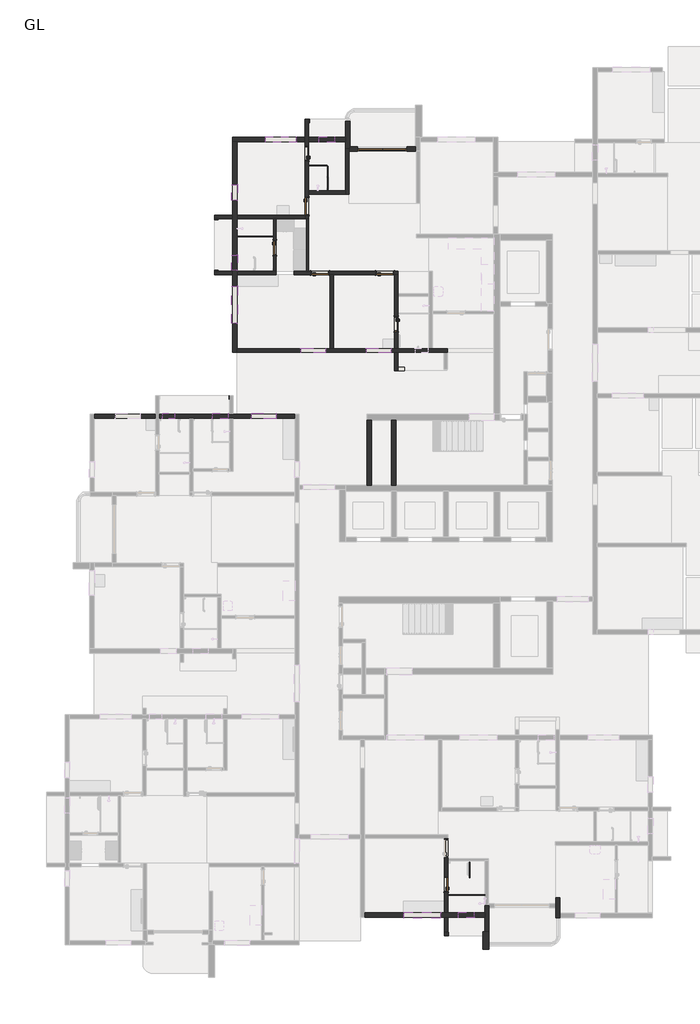
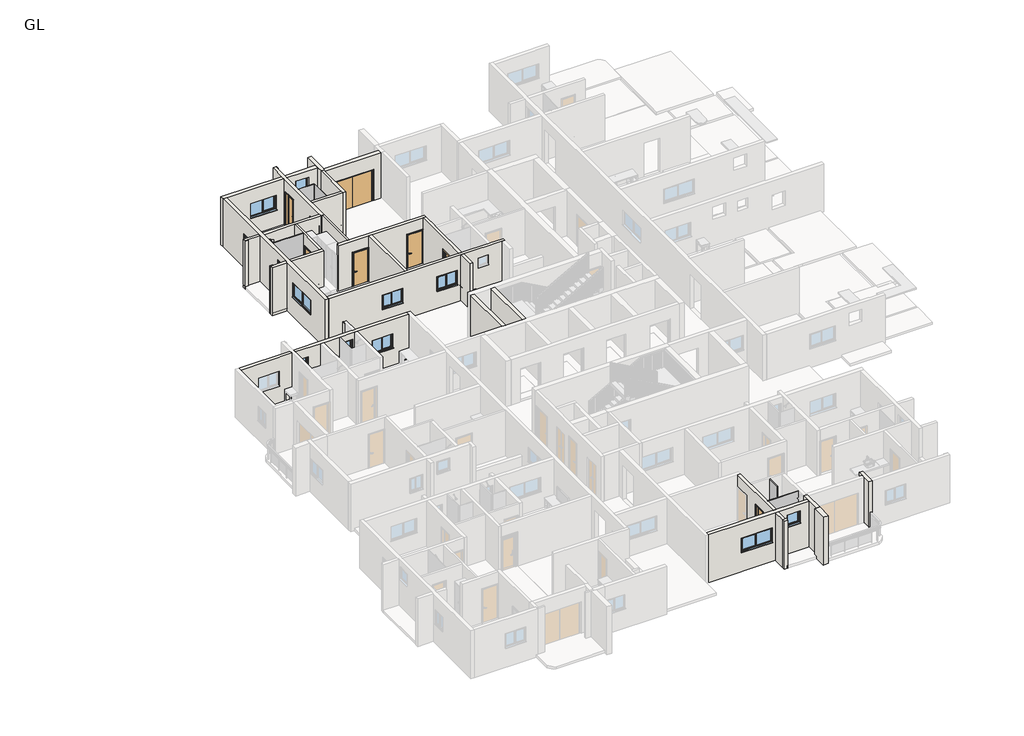
# One storey, part 3 of 14: 30 walls, 12 windows, 8 doors, 5 plates.
"""IFC4 building model written with IfcOpenShell, lengths in millimetres."""

from ifc_helpers import new_model, si_unit, frame, origin, origin_with_axes, place, context, project, spatial, polyline, outline, extrude, faceted_brep, transform, mapped, element, save
from components import doors_concept_extdbl_8_449e5563, doors_intsgl_2_5_door_ce04bd24, doors_intsgl_2_5_door_1f5f3f16, doors_intsgl_2_5_door_57e365e7, doors_intsgl_2_5_door_fd097d29, doors_intsgl_3_door_8261d8fb, system_panel_glazed_7a21471d, system_panel_glazed_bd0dc997, system_panel_glazed_f5f8a0d0, system_panel_glazed_29ba505a, system_panel_glazed_fbb400a4, windows_dbl_plain_2_5_5b7baf13, windows_dbl_plain_4_e08ba9e4, windows_dbl_plain_4_44133fe2, windows_dbl_plain_5_e9a2d570, windows_dbl_plain_6_3da2432f, windows_dbl_plain_6_22e4277a, windows_sgl_plain_2_82341a49, windows_sgl_plain_2_5_9e76a6e6, windows_sgl_plain_2_5_21186da1, windows_sgl_plain_2_5_1233c963

model = new_model("IFC4")

# Units and contexts
model_context = context("Model", 3, world=origin())
ifc_project = project(units=[si_unit("LENGTHUNIT", "METRE", prefix="MILLI")], contexts=[model_context])

# Site, building, storey
site = spatial("IfcSite", under=ifc_project)
building = spatial("IfcBuilding", under=site)
storey = spatial("IfcBuildingStorey", under=building, Name="GL", Elevation=0.0)

# Doors
placement = place(None, origin())
doors_concept_extdbl_8_shape = doors_concept_extdbl_8_449e5563(model_context)
element("IfcDoor", 1, ObjectType="Doors_Concept_ExtDbl : 8'", at=placement, inside=storey, context=model_context, shape_type="MappedRepresentation", body=[
    mapped(doors_concept_extdbl_8_shape, transform((-1155.7878137, 95616.8756254, 0.0), x_axis=(-1.0, 0.0, 0.0), y_axis=(0.0, -1.0, 0.0), z_axis=(0.0, 0.0, 1.0))),
])
doors_intsgl_2_5_door_shape = doors_intsgl_2_5_door_ce04bd24(model_context)
element("IfcDoor", 2, ObjectType="Doors_IntSgl : 2.5' DOOR", at=placement, inside=storey, context=model_context, shape_type="MappedRepresentation", body=[
    mapped(doors_intsgl_2_5_door_shape, transform((-457.962999, 86931.0916254, 149.9616), x_axis=(0.0, -1.0, 0.0), y_axis=(1.0, 0.0, 0.0), z_axis=(0.0, 0.0, 1.0))),
])
doors_intsgl_2_5_door_2_shape = doors_intsgl_2_5_door_1f5f3f16(model_context)
element("IfcDoor", 3, ObjectType="Doors_IntSgl : 2.5' DOOR", at=placement, inside=storey, context=model_context, shape_type="MappedRepresentation", body=[
    mapped(doors_intsgl_2_5_door_2_shape, transform((-6490.3162192, 90712.3517744, 149.9616), x_axis=(0.0, -1.0, 0.0), y_axis=(1.0, 0.0, 0.0), z_axis=(0.0, 0.0, 1.0))),
])
doors_intsgl_2_5_door_3_shape = doors_intsgl_2_5_door_57e365e7(model_context)
element("IfcDoor", 4, ObjectType="Doors_IntSgl : 2.5' DOOR", at=placement, inside=storey, context=model_context, shape_type="MappedRepresentation", body=[
    mapped(doors_intsgl_2_5_door_3_shape, transform((2014.4093567, 59142.1083045, 149.9616), x_axis=(0.0, 1.0, 0.0), y_axis=(-1.0, 0.0, 0.0), z_axis=(0.0, 0.0, 1.0))),
])
doors_intsgl_2_5_door_4_shape = doors_intsgl_2_5_door_fd097d29(model_context)
element("IfcDoor", 5, ObjectType="Doors_IntSgl : 2.5' DOOR", at=placement, inside=storey, context=model_context, shape_type="MappedRepresentation", body=[
    mapped(doors_intsgl_2_5_door_4_shape, transform((-4892.1482192, 95388.5507225, 149.9616), x_axis=(0.0, 1.0, 0.0), y_axis=(-1.0, 0.0, 0.0), z_axis=(0.0, 0.0, 1.0))),
])
doors_intsgl_3_door_shape = doors_intsgl_3_door_8261d8fb(model_context)
element("IfcDoor", 6, ObjectType="Doors_IntSgl : 3' DOOR", at=placement, inside=storey, context=model_context, shape_type="MappedRepresentation", body=[
    mapped(doors_intsgl_3_door_shape, transform((-1027.430999, 89469.7837744, 149.9616), x_axis=(1.0, 0.0, 0.0), y_axis=(0.0, 1.0, 0.0), z_axis=(0.0, 0.0, 1.0))),
])
element("IfcDoor", 7, ObjectType="Doors_IntSgl : 3' DOOR", at=placement, inside=storey, context=model_context, shape_type="MappedRepresentation", body=[
    mapped(doors_intsgl_3_door_shape, transform((-4246.4802192, 89469.7837744, 149.9616), x_axis=(1.0, 0.0, 0.0), y_axis=(0.0, 1.0, 0.0), z_axis=(0.0, 0.0, 1.0))),
])
element("IfcDoor", 8, ObjectType="Doors_IntSgl : 3' DOOR", at=placement, inside=storey, context=model_context, shape_type="MappedRepresentation", body=[
    mapped(doors_intsgl_3_door_shape, transform((-4892.1482192, 92780.648129, 149.9616), x_axis=(0.0, -1.0, 0.0), y_axis=(1.0, 0.0, 0.0), z_axis=(0.0, 0.0, 1.0))),
])

# Plates
system_panel_glazed_shape = system_panel_glazed_7a21471d(model_context)
element("IfcPlate", 9, ObjectType="System Panel : Glazed", at=placement, inside=storey, context=model_context, shape_type="MappedRepresentation", body=[
    mapped(system_panel_glazed_shape, transform((3014.0263567, 58649.9833045, 0.0), x_axis=(-1.0, 0.0, 0.0), y_axis=(0.0, -1.0, 0.0), z_axis=(0.0, 0.0, 1.0))),
])
system_panel_glazed_2_shape = system_panel_glazed_bd0dc997(model_context)
element("IfcPlate", 10, ObjectType="System Panel : Glazed", at=placement, inside=storey, context=model_context, shape_type="MappedRepresentation", body=[
    mapped(system_panel_glazed_2_shape, transform((3149.1144026, 59856.6583045, 0.0), x_axis=(0.0, -1.0, 0.0), y_axis=(1.0, 0.0, 0.0), z_axis=(0.0, 0.0, 1.0))),
])
system_panel_glazed_3_shape = system_panel_glazed_f5f8a0d0(model_context)
element("IfcPlate", 11, ObjectType="System Panel : Glazed", at=placement, inside=storey, context=model_context, shape_type="MappedRepresentation", body=[
    mapped(system_panel_glazed_3_shape, transform((-7453.4306091, 91235.312129, 0.0), x_axis=(1.0, 0.0, 0.0), y_axis=(0.0, 1.0, 0.0), z_axis=(0.0, 0.0, 1.0))),
])
system_panel_glazed_4_shape = system_panel_glazed_29ba505a(model_context)
element("IfcPlate", 12, ObjectType="System Panel : Glazed", at=placement, inside=storey, context=model_context, shape_type="MappedRepresentation", body=[
    mapped(system_panel_glazed_4_shape, transform((-4348.0802192, 94755.9639277, 0.0), x_axis=(1.0, 0.0, 0.0), y_axis=(0.0, 1.0, 0.0), z_axis=(0.0, 0.0, 1.0))),
])
system_panel_glazed_5_shape = system_panel_glazed_fbb400a4(model_context)
element("IfcPlate", 13, ObjectType="System Panel : Glazed", at=placement, inside=storey, context=model_context, shape_type="MappedRepresentation", body=[
    mapped(system_panel_glazed_5_shape, transform((-3890.8802192, 94151.5180788, 0.0), x_axis=(0.0, -1.0, 0.0), y_axis=(1.0, 0.0, 0.0), z_axis=(0.0, 0.0, 1.0))),
])

# Walls
element("IfcWall", 14, ObjectType="W2", at=placement, inside=storey, context=model_context, shape_type="Brep", body=[
    faceted_brep([(-2987.294999, 95616.8756254, 0.0), (-2987.294999, 93547.0722299, 0.0), (-2987.294999, 93373.3362299, 0.0), (-2987.294999, 93373.3362299, 3000.0), (-2987.294999, 93547.0722299, 3000.0), (-2987.294999, 95616.8756254, 3000.0), (-2813.558999, 95616.8756254, 0.0), (-2813.558999, 95616.8756254, 3000.0), (-2813.558999, 95510.1956254, 3000.0), (-2813.558999, 93373.3362299, 3000.0), (-2813.558999, 93373.3362299, 0.0), (-2813.558999, 95510.1956254, 0.0)], [[[0, 1, 2, 3, 4, 5]], [[6, 7, 8, 9, 10, 11]], [[2, 1, 0, 6, 11, 10]], [[5, 4, 3, 9, 8, 7]], [[0, 5, 7, 6]], [[3, 2, 10, 9]]]),
])
element("IfcWall", 15, ObjectType="W2", at=placement, inside=storey, context=model_context, shape_type="Brep", body=[
    faceted_brep([(-4979.0162192, 97086.2867225, 0.0), (-4979.0162192, 96193.4556254, 0.0), (-4979.0162192, 95964.8556254, 0.0), (-4979.0162192, 92323.448129, 0.0), (-4979.0162192, 92149.712129, 0.0), (-4979.0162192, 92149.712129, 3000.0), (-4979.0162192, 92323.448129, 3000.0), (-4979.0162192, 95964.8556254, 3000.0), (-4979.0162192, 96193.4556254, 3000.0), (-4979.0162192, 97086.2867225, 3000.0), (-4979.0162192, 92323.448129, 2259.9616), (-4979.0162192, 92323.448129, 149.9616), (-4979.0162192, 93237.848129, 149.9616), (-4979.0162192, 93237.848129, 2259.9616), (-4979.0162192, 95769.5507225, 149.9616), (-4979.0162192, 95769.5507225, 2259.9616), (-4979.0162192, 95007.5507225, 2259.9616), (-4979.0162192, 95007.5507225, 149.9616), (-4805.2802192, 92149.712129, 0.0), (-4805.2802192, 93373.3362299, 0.0), (-4805.2802192, 93547.0722299, 0.0), (-4805.2802192, 95964.8556254, 0.0), (-4805.2802192, 96193.4556254, 0.0), (-4805.2802192, 96912.5507225, 0.0), (-4805.2802192, 97086.2867225, 0.0), (-4805.2802192, 97086.2867225, 3000.0), (-4805.2802192, 96912.5507225, 3000.0), (-4805.2802192, 96193.4556254, 3000.0), (-4805.2802192, 95964.8556254, 3000.0), (-4805.2802192, 93547.0722299, 3000.0), (-4805.2802192, 93373.3362299, 3000.0), (-4805.2802192, 92149.712129, 3000.0), (-4805.2802192, 92323.448129, 149.9616), (-4805.2802192, 92323.448129, 2259.9616), (-4805.2802192, 93237.848129, 2259.9616), (-4805.2802192, 93237.848129, 149.9616), (-4805.2802192, 95769.5507225, 2259.9616), (-4805.2802192, 95769.5507225, 149.9616), (-4805.2802192, 95007.5507225, 149.9616), (-4805.2802192, 95007.5507225, 2259.9616), (-4919.5802192, 92149.712129, 0.0), (-4919.5802192, 92149.712129, 3000.0)], [[[0, 1, 2, 3, 4, 5, 6, 7, 8, 9], [10, 11, 12, 13], [14, 15, 16, 17]], [[18, 19, 20, 21, 22, 23, 24, 25, 26, 27, 28, 29, 30, 31], [32, 33, 34, 35], [36, 37, 38, 39]], [[4, 3, 2, 1, 0, 24, 23, 22, 21, 20, 19, 18, 40]], [[9, 8, 7, 6, 5, 41, 31, 30, 29, 28, 27, 26, 25]], [[5, 4, 40, 18, 31, 41]], [[0, 9, 25, 24]], [[32, 11, 10, 33]], [[33, 10, 13, 34]], [[34, 13, 12, 35]], [[11, 32, 35, 12]], [[14, 37, 36, 15]], [[15, 36, 39, 16]], [[38, 17, 16, 39]], [[37, 14, 17, 38]]]),
])
element("IfcWall", 16, ObjectType="W2", at=placement, inside=storey, context=model_context, shape_type="Brep", body=[
    faceted_brep([(-8359.394999, 85538.1556254, 0.0), (-538.480999, 85538.1556254, 0.0), (-364.744999, 85538.1556254, 0.0), (1899.919001, 85538.1556254, 0.0), (2073.655001, 85538.1556254, 0.0), (2080.005001, 85538.1556254, 0.0), (2080.005001, 85538.1556254, 1171.2), (2080.005001, 85538.1556254, 3000.0), (2073.655001, 85538.1556254, 3000.0), (1899.919001, 85538.1556254, 3000.0), (-364.744999, 85538.1556254, 3000.0), (-538.480999, 85538.1556254, 3000.0), (-8359.394999, 85538.1556254, 3000.0), (-3962.5906208, 85538.1556254, 2110.0), (-3962.5906208, 85538.1556254, 1200.0), (-5181.7906208, 85538.1556254, 1200.0), (-5181.7906208, 85538.1556254, 2110.0), (-722.630999, 85538.1556254, 2110.0), (-722.630999, 85538.1556254, 1200.0), (-1941.830999, 85538.1556254, 1200.0), (-1941.830999, 85538.1556254, 2110.0), (1106.169001, 85538.1556254, 2438.4), (1106.169001, 85538.1556254, 1828.8), (496.569001, 85538.1556254, 1828.8), (496.569001, 85538.1556254, 2438.4), (-8359.394999, 85711.8916254, 0.0), (-8359.394999, 85711.8916254, 3000.0), (-3759.3906208, 85711.8916254, 3000.0), (-3585.6546208, 85711.8916254, 3000.0), (-544.830999, 85711.8916254, 3000.0), (-371.094999, 85711.8916254, 3000.0), (1156.969001, 85711.8916254, 3000.0), (1330.705001, 85711.8916254, 3000.0), (2080.005001, 85711.8916254, 3000.0), (2080.005001, 85711.8916254, 1171.2), (2080.005001, 85711.8916254, 0.0), (1330.705001, 85711.8916254, 0.0), (1156.969001, 85711.8916254, 0.0), (-371.094999, 85711.8916254, 0.0), (-544.830999, 85711.8916254, 0.0), (-3585.6546208, 85711.8916254, 0.0), (-3759.3906208, 85711.8916254, 0.0), (-3962.5906208, 85711.8916254, 2110.0), (-5181.7906208, 85711.8916254, 2110.0), (-5181.7906208, 85711.8916254, 1200.0), (-3962.5906208, 85711.8916254, 1200.0), (-722.630999, 85711.8916254, 2110.0), (-1941.830999, 85711.8916254, 2110.0), (-1941.830999, 85711.8916254, 1200.0), (-722.630999, 85711.8916254, 1200.0), (1106.169001, 85711.8916254, 2438.4), (496.569001, 85711.8916254, 2438.4), (496.569001, 85711.8916254, 1828.8), (1106.169001, 85711.8916254, 1828.8)], [[[0, 1, 2, 3, 4, 5, 6, 7, 8, 9, 10, 11, 12], [13, 14, 15, 16], [17, 18, 19, 20], [21, 22, 23, 24]], [[25, 26, 27, 28, 29, 30, 31, 32, 33, 34, 35, 36, 37, 38, 39, 40, 41], [42, 43, 44, 45], [46, 47, 48, 49], [50, 51, 52, 53]], [[5, 4, 3, 2, 1, 0, 25, 41, 40, 39, 38, 37, 36, 35]], [[7, 6, 5, 35, 34, 33]], [[12, 11, 10, 9, 8, 7, 33, 32, 31, 30, 29, 28, 27, 26]], [[0, 12, 26, 25]], [[14, 13, 42, 45]], [[15, 14, 45, 44]], [[16, 15, 44, 43]], [[13, 16, 43, 42]], [[18, 17, 46, 49]], [[19, 18, 49, 48]], [[20, 19, 48, 47]], [[17, 20, 47, 46]], [[22, 21, 50, 53]], [[23, 22, 53, 52]], [[24, 23, 52, 51]], [[21, 24, 51, 50]]]),
])
element("IfcWall", 17, ObjectType="W2", at=placement, inside=storey, context=model_context, shape_type="SweptSolid", body=[
    extrude(outline(polyline([(-4805.2802192, 93547.0722299), (-2987.294999, 93547.0722299), (-2987.294999, 93373.3362299), (-4805.2802192, 93373.3362299), (-4805.2802192, 93547.0722299)])), origin_with_axes(), (0.0, 0.0, 1.0), 3000.0),
])
element("IfcWall", 18, ObjectType="W2", at=placement, inside=storey, context=model_context, shape_type="Brep", body=[
    faceted_brep([(-4979.0162192, 92323.448129, 3000.0), (-4979.0162192, 92323.448129, 0.0), (-8359.394999, 92323.448129, 0.0), (-8359.394999, 92323.448129, 3000.0), (-4979.0162192, 92149.712129, 0.0), (-4979.0162192, 92149.712129, 3000.0), (-6433.1662192, 92149.712129, 3000.0), (-6547.4662192, 92149.712129, 3000.0), (-8359.394999, 92149.712129, 3000.0), (-8359.394999, 92149.712129, 0.0), (-6547.4662192, 92149.712129, 0.0), (-6433.1662192, 92149.712129, 0.0)], [[[0, 1, 2, 3]], [[4, 5, 6, 7, 8, 9, 10, 11]], [[1, 4, 11, 10, 9, 2]], [[5, 0, 3, 8, 7, 6]], [[1, 0, 5, 4]], [[3, 2, 9, 8]]]),
    faceted_brep([(-9487.5162192, 92323.448129, 0.0), (-9487.5162192, 92323.448129, 3000.0), (-8587.994999, 92323.448129, 3000.0), (-8587.994999, 92323.448129, 0.0), (-9487.5162192, 92149.712129, 3000.0), (-9487.5162192, 92149.712129, 0.0), (-9313.7802192, 92149.712129, 0.0), (-8587.994999, 92149.712129, 0.0), (-8587.994999, 92149.712129, 3000.0), (-9313.7802192, 92149.712129, 3000.0)], [[[0, 1, 2, 3]], [[4, 5, 6, 7, 8, 9]], [[5, 0, 3, 7, 6]], [[1, 4, 9, 8, 2]], [[3, 2, 8, 7]], [[1, 0, 5, 4]]]),
])
element("IfcWall", 19, ObjectType="W2", at=placement, inside=storey, context=model_context, shape_type="Brep", body=[
    faceted_brep([(-9487.5162192, 89382.9157744, 3000.0), (-9487.5162192, 89382.9157744, 0.0), (-8587.994999, 89382.9157744, 0.0), (-8587.994999, 89382.9157744, 3000.0), (-9487.5162192, 89556.6517744, 0.0), (-9487.5162192, 89556.6517744, 3000.0), (-9313.7802192, 89556.6517744, 3000.0), (-8587.994999, 89556.6517744, 3000.0), (-8587.994999, 89556.6517744, 0.0), (-9313.7802192, 89556.6517744, 0.0)], [[[0, 1, 2, 3]], [[4, 5, 6, 7, 8, 9]], [[1, 4, 9, 8, 2]], [[5, 0, 3, 7, 6]], [[3, 2, 8, 7]], [[1, 0, 5, 4]]]),
    faceted_brep([(-6433.1662192, 89382.9157744, 0.0), (-6433.1662192, 89382.9157744, 3000.0), (-8359.394999, 89382.9157744, 3000.0), (-8359.394999, 89382.9157744, 0.0), (-6433.1662192, 89556.6517744, 3000.0), (-6433.1662192, 89556.6517744, 0.0), (-6547.4662192, 89556.6517744, 0.0), (-8359.394999, 89556.6517744, 0.0), (-8359.394999, 89556.6517744, 3000.0), (-6547.4662192, 89556.6517744, 3000.0)], [[[0, 1, 2, 3]], [[4, 5, 6, 7, 8, 9]], [[5, 0, 3, 7, 6]], [[1, 4, 9, 8, 2]], [[3, 2, 8, 7]], [[1, 0, 5, 4]]]),
])
element("IfcWall", 20, ObjectType="W2", at=placement, inside=storey, context=model_context, shape_type="SweptSolid", body=[
    extrude(outline(polyline([(-9487.5162192, 92111.612129), (-9487.5162192, 92149.712129), (-9313.7802192, 92149.712129), (-9313.7802192, 92111.612129), (-9487.5162192, 92111.612129)])), origin_with_axes(), (0.0, 0.0, 1.0), 3000.0),
])
element("IfcWall", 21, ObjectType="W2", at=placement, inside=storey, context=model_context, shape_type="SweptSolid", body=[
    extrude(outline(polyline([(-9487.5162192, 89556.6517744), (-9487.5162192, 89601.1017744), (-9313.7802192, 89601.1017744), (-9313.7802192, 89556.6517744), (-9487.5162192, 89556.6517744)])), origin_with_axes(), (0.0, 0.0, 1.0), 3000.0),
])
element("IfcWall", 22, ObjectType="W2", at=placement, inside=storey, context=model_context, shape_type="Brep", body=[
    faceted_brep([(-5531.8235062, 89382.9157744, 0.0), (-3759.3906208, 89382.9157744, 0.0), (-3585.6546208, 89382.9157744, 0.0), (-544.830999, 89382.9157744, 0.0), (-371.094999, 89382.9157744, 0.0), (-371.094999, 89382.9157744, 3000.0), (-544.830999, 89382.9157744, 3000.0), (-3585.6546208, 89382.9157744, 3000.0), (-3759.3906208, 89382.9157744, 3000.0), (-5531.8235062, 89382.9157744, 3000.0), (-570.230999, 89382.9157744, 2259.9616), (-570.230999, 89382.9157744, 149.9616), (-1484.630999, 89382.9157744, 149.9616), (-1484.630999, 89382.9157744, 2259.9616), (-3789.2802192, 89382.9157744, 2259.9616), (-3789.2802192, 89382.9157744, 149.9616), (-4703.6802192, 89382.9157744, 149.9616), (-4703.6802192, 89382.9157744, 2259.9616), (-371.094999, 89556.6517744, 0.0), (-4805.2802192, 89556.6517744, 0.0), (-4919.5802192, 89556.6517744, 0.0), (-5531.8235062, 89556.6517744, 0.0), (-5531.8235062, 89556.6517744, 3000.0), (-4919.5802192, 89556.6517744, 3000.0), (-4805.2802192, 89556.6517744, 3000.0), (-371.094999, 89556.6517744, 3000.0), (-570.230999, 89556.6517744, 149.9616), (-570.230999, 89556.6517744, 2259.9616), (-1484.630999, 89556.6517744, 2259.9616), (-1484.630999, 89556.6517744, 149.9616), (-3789.2802192, 89556.6517744, 149.9616), (-3789.2802192, 89556.6517744, 2259.9616), (-4703.6802192, 89556.6517744, 2259.9616), (-4703.6802192, 89556.6517744, 149.9616)], [[[0, 1, 2, 3, 4, 5, 6, 7, 8, 9], [10, 11, 12, 13], [14, 15, 16, 17]], [[18, 19, 20, 21, 22, 23, 24, 25], [26, 27, 28, 29], [30, 31, 32, 33]], [[4, 3, 2, 1, 0, 21, 20, 19, 18]], [[9, 8, 7, 6, 5, 25, 24, 23, 22]], [[0, 9, 22, 21]], [[5, 4, 18, 25]], [[26, 11, 10, 27]], [[27, 10, 13, 28]], [[12, 29, 28, 13]], [[11, 26, 29, 12]], [[30, 15, 14, 31]], [[31, 14, 17, 32]], [[32, 17, 16, 33]], [[15, 30, 33, 16]]]),
])
element("IfcWall", 23, ObjectType="W2", at=placement, inside=storey, context=model_context, shape_type="SweptSolid", body=[
    extrude(outline(polyline([(-3585.6546208, 89382.9157744), (-3585.6546208, 85711.8916254), (-3759.3906208, 85711.8916254), (-3759.3906208, 89382.9157744), (-3585.6546208, 89382.9157744)])), origin_with_axes(), (0.0, 0.0, 1.0), 3000.0),
])
element("IfcWall", 24, ObjectType="W2", at=placement, inside=storey, context=model_context, shape_type="Brep", body=[
    faceted_brep([(-371.094999, 85711.8916254, 0.0), (-371.094999, 88321.7416254, 0.0), (-371.094999, 88436.0416254, 0.0), (-371.094999, 89382.9157744, 0.0), (-371.094999, 89382.9157744, 3000.0), (-371.094999, 88436.0416254, 3000.0), (-371.094999, 88321.7416254, 3000.0), (-371.094999, 85711.8916254, 3000.0), (-371.094999, 86550.0916254, 149.9616), (-371.094999, 86550.0916254, 2259.9616), (-371.094999, 87312.0916254, 2259.9616), (-371.094999, 87312.0916254, 149.9616), (-544.830999, 89382.9157744, 0.0), (-544.830999, 85711.8916254, 0.0), (-544.830999, 85711.8916254, 3000.0), (-544.830999, 89382.9157744, 3000.0), (-544.830999, 86550.0916254, 2259.9616), (-544.830999, 86550.0916254, 149.9616), (-544.830999, 87312.0916254, 149.9616), (-544.830999, 87312.0916254, 2259.9616)], [[[0, 1, 2, 3, 4, 5, 6, 7], [8, 9, 10, 11]], [[12, 13, 14, 15], [16, 17, 18, 19]], [[3, 2, 1, 0, 13, 12]], [[7, 6, 5, 4, 15, 14]], [[0, 7, 14, 13]], [[4, 3, 12, 15]], [[8, 17, 16, 9]], [[9, 16, 19, 10]], [[10, 19, 18, 11]], [[17, 8, 11, 18]]]),
])
element("IfcWall", 25, ObjectType="W2", at=placement, inside=storey, context=model_context, shape_type="Brep", body=[
    faceted_brep([(-538.480999, 85538.1556254, 0.0), (-538.480999, 84611.0556254, 0.0), (-538.480999, 84611.0556254, 3000.0), (-538.480999, 85538.1556254, 3000.0), (-364.744999, 85538.1556254, 0.0), (-364.744999, 85538.1556254, 3000.0), (-364.744999, 84611.0556254, 3000.0), (-364.744999, 84611.0556254, 1171.2), (-364.744999, 84611.0556254, 0.0), (-364.744999, 84784.7916254, 0.0)], [[[0, 1, 2, 3]], [[4, 5, 6, 7, 8, 9]], [[1, 0, 4, 9, 8]], [[3, 2, 6, 5]], [[0, 3, 5, 4]], [[2, 1, 8, 7, 6]]]),
])
element("IfcWall", 26, ObjectType="W2", at=placement, inside=storey, context=model_context, shape_type="SweptSolid", body=[
    extrude(outline(polyline([(-66.294999, 84611.0556254), (-364.744999, 84611.0556254), (-364.744999, 84784.7916254), (-66.294999, 84784.7916254), (-66.294999, 84611.0556254)])), origin_with_axes(), (0.0, 0.0, 1.0), 1171.2),
])
element("IfcWall", 27, ObjectType="W2", at=placement, inside=storey, context=model_context, shape_type="SweptSolid", body=[
    extrude(outline(polyline([(-8762.4991708, 83367.762856), (-8724.3991708, 83367.762856), (-8724.3991708, 83194.026856), (-8762.4991708, 83194.026856), (-8762.4991708, 83367.762856)])), origin_with_axes(), (0.0, 0.0, 1.0), 3000.0),
])
element("IfcWall", 28, ObjectType="W2", at=placement, inside=storey, context=model_context, shape_type="SweptSolid", body=[
    extrude(outline(polyline([(-4773.5302192, 96912.5507225), (-4805.2802192, 96912.5507225), (-4805.2802192, 97086.2867225), (-4773.5302192, 97086.2867225), (-4773.5302192, 96912.5507225)])), origin_with_axes(), (0.0, 0.0, 1.0), 3000.0),
])
element("IfcWall", 29, ObjectType="W2", at=placement, inside=storey, context=model_context, shape_type="Brep", body=[
    faceted_brep([(1930.5893567, 56602.5684195, 0.0), (2136.3293567, 56602.5684195, 0.0), (2136.3293567, 56602.5684195, 3000.0), (1930.5893567, 56602.5684195, 3000.0), (1930.5893567, 56776.3044195, 0.0), (1930.5893567, 56776.3044195, 3000.0), (2098.2293567, 56776.3044195, 3000.0), (2136.3293567, 56776.3044195, 3000.0), (2136.3293567, 56776.3044195, 0.0), (2098.2293567, 56776.3044195, 0.0)], [[[0, 1, 2, 3]], [[4, 5, 6, 7, 8, 9]], [[1, 0, 4, 9, 8]], [[2, 1, 8, 7]], [[3, 2, 7, 6, 5]], [[0, 3, 5, 4]]]),
])
element("IfcWall", 30, ObjectType="W3", at=placement, inside=storey, context=model_context, shape_type="SweptSolid", body=[
    extrude(outline(polyline([(-4919.5802192, 89556.6517744), (-4919.5802192, 92149.712129), (-4805.2802192, 92149.712129), (-4805.2802192, 89556.6517744), (-4919.5802192, 89556.6517744)])), origin_with_axes(), (0.0, 0.0, 1.0), 3000.0),
])
element("IfcWall", 31, ObjectType="W3", at=placement, inside=storey, context=model_context, shape_type="SweptSolid", body=[
    extrude(outline(polyline([(92149.712129, 0.0), (89556.6517744, 0.0), (89556.6517744, 3000.0), (92149.712129, 3000.0), (92149.712129, 0.0)]), holes=[polyline([(90331.3517744, 2259.9616), (90331.3517744, 149.9616), (91093.3517744, 149.9616), (91093.3517744, 2259.9616), (90331.3517744, 2259.9616)])]), frame((-6547.4662192, 0.0, 0.0), z_axis=(1.0, 0.0, 0.0), x_axis=(0.0, 1.0, 0.0)), (0.0, 0.0, 1.0), 114.3),
])
element("IfcWall", 32, ObjectType="W4", at=placement, inside=storey, context=model_context, shape_type="Brep", body=[
    faceted_brep([(4143.1833567, 55914.0279605, 0.0), (4143.1833567, 56803.0279605, 0.0), (4143.1833567, 56803.0279605, 3000.0), (4143.1833567, 55914.0279605, 3000.0), (3838.3833567, 55914.0279605, 0.0), (3838.3833567, 55914.0279605, 3000.0), (3838.3833567, 56803.0279605, 3000.0), (3838.3833567, 56803.0279605, 0.0), (3929.8233567, 56803.0279605, 0.0), (3929.8233567, 56803.0279605, 3000.0)], [[[0, 1, 2, 3]], [[4, 5, 6, 7]], [[1, 0, 4, 7, 8]], [[2, 1, 8, 7, 6, 9]], [[3, 2, 9, 6, 5]], [[0, 3, 5, 4]]]),
])
element("IfcWall", 33, ObjectType="W5", at=placement, inside=storey, context=model_context, shape_type="Brep", body=[
    faceted_brep([(-2987.294999, 96999.4187225, 0.0), (-2987.294999, 96193.4556254, 0.0), (-2987.294999, 95964.8556254, 0.0), (-2987.294999, 95616.8756254, 0.0), (-2987.294999, 95616.8756254, 3000.0), (-2987.294999, 95964.8556254, 3000.0), (-2987.294999, 96193.4556254, 3000.0), (-2987.294999, 96999.4187225, 3000.0), (-2758.694999, 96999.4187225, 0.0), (-2758.694999, 96999.4187225, 3000.0), (-2758.694999, 95723.5556254, 3000.0), (-2758.694999, 95616.8756254, 3000.0), (-2758.694999, 95616.8756254, 0.0), (-2758.694999, 95723.5556254, 0.0), (-2813.558999, 95616.8756254, 0.0), (-2813.558999, 95616.8756254, 3000.0)], [[[0, 1, 2, 3, 4, 5, 6, 7]], [[8, 9, 10, 11, 12, 13]], [[3, 2, 1, 0, 8, 13, 12, 14]], [[4, 3, 14, 12, 11, 15]], [[7, 6, 5, 4, 15, 11, 10, 9]], [[0, 7, 9, 8]]]),
])
element("IfcWall", 34, ObjectType="W5", at=placement, inside=storey, context=model_context, shape_type="Brep", body=[
    faceted_brep([(-2987.294999, 96193.4556254, 3000.0), (-2987.294999, 96193.4556254, 0.0), (-4805.2802192, 96193.4556254, 0.0), (-4805.2802192, 96193.4556254, 3000.0), (-4282.694999, 96193.4556254, 2590.8), (-4282.694999, 96193.4556254, 1828.8), (-3520.694999, 96193.4556254, 1828.8), (-3520.694999, 96193.4556254, 2590.8), (-2987.294999, 95964.8556254, 0.0), (-2987.294999, 95964.8556254, 3000.0), (-4805.2802192, 95964.8556254, 3000.0), (-4805.2802192, 95964.8556254, 0.0), (-4282.694999, 95964.8556254, 1828.8), (-4282.694999, 95964.8556254, 2590.8), (-3520.694999, 95964.8556254, 2590.8), (-3520.694999, 95964.8556254, 1828.8)], [[[0, 1, 2, 3], [4, 5, 6, 7]], [[8, 9, 10, 11], [12, 13, 14, 15]], [[1, 8, 11, 2]], [[9, 0, 3, 10]], [[1, 0, 9, 8]], [[3, 2, 11, 10]], [[5, 4, 13, 12]], [[6, 5, 12, 15]], [[7, 6, 15, 14]], [[4, 7, 14, 13]]]),
    faceted_brep([(-8587.994999, 96193.4556254, 0.0), (-8587.994999, 96193.4556254, 3000.0), (-4979.0162192, 96193.4556254, 3000.0), (-4979.0162192, 96193.4556254, 0.0), (-6949.694999, 96193.4556254, 2110.0), (-6949.694999, 96193.4556254, 1200.0), (-5425.694999, 96193.4556254, 1200.0), (-5425.694999, 96193.4556254, 2110.0), (-8587.994999, 95964.8556254, 3000.0), (-8587.994999, 95964.8556254, 0.0), (-8359.394999, 95964.8556254, 0.0), (-4979.0162192, 95964.8556254, 0.0), (-4979.0162192, 95964.8556254, 3000.0), (-8359.394999, 95964.8556254, 3000.0), (-6949.694999, 95964.8556254, 1200.0), (-6949.694999, 95964.8556254, 2110.0), (-5425.694999, 95964.8556254, 2110.0), (-5425.694999, 95964.8556254, 1200.0)], [[[0, 1, 2, 3], [4, 5, 6, 7]], [[8, 9, 10, 11, 12, 13], [14, 15, 16, 17]], [[9, 0, 3, 11, 10]], [[1, 8, 13, 12, 2]], [[3, 2, 12, 11]], [[1, 0, 9, 8]], [[5, 4, 15, 14]], [[6, 5, 14, 17]], [[7, 6, 17, 16]], [[4, 7, 16, 15]]]),
])
element("IfcWall", 35, ObjectType="W5", at=placement, inside=storey, context=model_context, shape_type="Brep", body=[
    faceted_brep([(-8587.994999, 95964.8556254, 0.0), (-8587.994999, 92323.448129, 0.0), (-8587.994999, 92149.712129, 0.0), (-8587.994999, 89556.6517744, 0.0), (-8587.994999, 89382.9157744, 0.0), (-8587.994999, 85538.1556254, 0.0), (-8587.994999, 85538.1556254, 3000.0), (-8587.994999, 89382.9157744, 3000.0), (-8587.994999, 89556.6517744, 3000.0), (-8587.994999, 92149.712129, 3000.0), (-8587.994999, 92323.448129, 3000.0), (-8587.994999, 95964.8556254, 3000.0), (-8587.994999, 93069.2556254, 2110.0), (-8587.994999, 93069.2556254, 1200.0), (-8587.994999, 93831.2556254, 1200.0), (-8587.994999, 93831.2556254, 2110.0), (-8587.994999, 89589.4556254, 2590.8), (-8587.994999, 89589.4556254, 1828.8), (-8587.994999, 90351.4556254, 1828.8), (-8587.994999, 90351.4556254, 2590.8), (-8587.994999, 86973.2556254, 2110.0), (-8587.994999, 86973.2556254, 1200.0), (-8587.994999, 88802.0556254, 1200.0), (-8587.994999, 88802.0556254, 2110.0), (-8359.394999, 95964.8556254, 0.0), (-8359.394999, 95964.8556254, 3000.0), (-8359.394999, 92323.448129, 3000.0), (-8359.394999, 92149.712129, 3000.0), (-8359.394999, 89556.6517744, 3000.0), (-8359.394999, 89382.9157744, 3000.0), (-8359.394999, 85711.8916254, 3000.0), (-8359.394999, 85538.1556254, 3000.0), (-8359.394999, 85538.1556254, 0.0), (-8359.394999, 85711.8916254, 0.0), (-8359.394999, 89382.9157744, 0.0), (-8359.394999, 89556.6517744, 0.0), (-8359.394999, 92149.712129, 0.0), (-8359.394999, 92323.448129, 0.0), (-8359.394999, 93069.2556254, 2110.0), (-8359.394999, 93831.2556254, 2110.0), (-8359.394999, 93831.2556254, 1200.0), (-8359.394999, 93069.2556254, 1200.0), (-8359.394999, 89589.4556254, 2590.8), (-8359.394999, 90351.4556254, 2590.8), (-8359.394999, 90351.4556254, 1828.8), (-8359.394999, 89589.4556254, 1828.8), (-8359.394999, 86973.2556254, 2110.0), (-8359.394999, 88802.0556254, 2110.0), (-8359.394999, 88802.0556254, 1200.0), (-8359.394999, 86973.2556254, 1200.0)], [[[0, 1, 2, 3, 4, 5, 6, 7, 8, 9, 10, 11], [12, 13, 14, 15], [16, 17, 18, 19], [20, 21, 22, 23]], [[24, 25, 26, 27, 28, 29, 30, 31, 32, 33, 34, 35, 36, 37], [38, 39, 40, 41], [42, 43, 44, 45], [46, 47, 48, 49]], [[5, 4, 3, 2, 1, 0, 24, 37, 36, 35, 34, 33, 32]], [[11, 10, 9, 8, 7, 6, 31, 30, 29, 28, 27, 26, 25]], [[0, 11, 25, 24]], [[6, 5, 32, 31]], [[13, 12, 38, 41]], [[14, 13, 41, 40]], [[15, 14, 40, 39]], [[12, 15, 39, 38]], [[17, 16, 42, 45]], [[18, 17, 45, 44]], [[19, 18, 44, 43]], [[16, 19, 43, 42]], [[21, 20, 46, 49]], [[22, 21, 49, 48]], [[23, 22, 48, 47]], [[20, 23, 47, 46]]]),
])
element("IfcWall", 36, ObjectType="W7", at=placement, inside=storey, context=model_context, shape_type="SweptSolid", body=[
    extrude(outline(polyline([(-1903.3131613, 78948.3487724), (-1903.3131613, 82157.7073985), (-1680.8091613, 82157.7073985), (-1680.8091613, 78948.3487724), (-1903.3131613, 78948.3487724)])), origin_with_axes(), (0.0, 0.0, 1.0), 3000.0),
])
element("IfcWall", 37, ObjectType="W7", at=placement, inside=storey, context=model_context, shape_type="SweptSolid", body=[
    extrude(outline(polyline([(-701.1311613, 78948.3487724), (-701.1311613, 82157.7073985), (-478.6271613, 82157.7073985), (-478.6271613, 78948.3487724), (-701.1311613, 78948.3487724)])), origin_with_axes(), (0.0, 0.0, 1.0), 3000.0),
])
element("IfcWall", 38, ObjectType="W8", at=placement, inside=storey, context=model_context, shape_type="Brep", body=[
    faceted_brep([(-2374.9878137, 95723.5556254, 2110.0), (-2374.9878137, 95723.5556254, 0.0), (-2758.694999, 95723.5556254, 0.0), (-2758.694999, 95723.5556254, 3000.0), (501.9833716, 95723.5556254, 3000.0), (501.9833716, 95723.5556254, 0.0), (63.4121863, 95723.5556254, 0.0), (63.4121863, 95723.5556254, 2110.0), (-2813.558999, 95510.1956254, 0.0), (-2374.9878137, 95510.1956254, 0.0), (-2374.9878137, 95510.1956254, 2110.0), (63.4121863, 95510.1956254, 2110.0), (63.4121863, 95510.1956254, 0.0), (501.9833716, 95510.1956254, 0.0), (501.9833716, 95510.1956254, 3000.0), (-2813.558999, 95510.1956254, 3000.0), (-2813.558999, 95616.8756254, 0.0), (-2758.694999, 95616.8756254, 0.0), (-2758.694999, 95616.8756254, 3000.0), (-2813.558999, 95616.8756254, 3000.0)], [[[0, 1, 2, 3, 4, 5, 6, 7]], [[8, 9, 10, 11, 12, 13, 14, 15]], [[6, 5, 13, 12]], [[2, 1, 9, 8, 16, 17]], [[4, 3, 18, 19, 15, 14]], [[5, 4, 14, 13]], [[3, 2, 17, 18]], [[17, 16, 19, 18]], [[16, 8, 15, 19]], [[12, 11, 7, 6]], [[10, 9, 1, 0]], [[11, 10, 0, 7]]]),
])
element("IfcWall", 39, ObjectType="W8", at=placement, inside=storey, context=model_context, shape_type="Brep", body=[
    faceted_brep([(-2044.3665436, 57509.8965193, 0.0), (1930.5893567, 57509.8965193, 0.0), (2098.2293567, 57509.8965193, 0.0), (3929.8233567, 57509.8965193, 0.0), (3929.8233567, 57509.8965193, 3000.0), (2098.2293567, 57509.8965193, 3000.0), (1930.5893567, 57509.8965193, 3000.0), (-2044.3665436, 57509.8965193, 3000.0), (1740.2334564, 57509.8965193, 2110.0), (1740.2334564, 57509.8965193, 1200.0), (-88.5665436, 57509.8965193, 1200.0), (-88.5665436, 57509.8965193, 2110.0), (2634.4233567, 57509.8965193, 2590.8), (3396.4233567, 57509.8965193, 2590.8), (3396.4233567, 57509.8965193, 1828.8), (2634.4233567, 57509.8965193, 1828.8), (-2044.3665436, 57723.2565193, 0.0), (-2044.3665436, 57723.2565193, 3000.0), (1930.5893567, 57723.2565193, 3000.0), (2098.2293567, 57723.2565193, 3000.0), (3929.8233567, 57723.2565193, 3000.0), (3929.8233567, 57723.2565193, 0.0), (2098.2293567, 57723.2565193, 0.0), (1930.5893567, 57723.2565193, 0.0), (1740.2334564, 57723.2565193, 2110.0), (-88.5665436, 57723.2565193, 2110.0), (-88.5665436, 57723.2565193, 1200.0), (1740.2334564, 57723.2565193, 1200.0), (2634.4233567, 57723.2565193, 2590.8), (2634.4233567, 57723.2565193, 1828.8), (3396.4233567, 57723.2565193, 1828.8), (3396.4233567, 57723.2565193, 2590.8)], [[[0, 1, 2, 3, 4, 5, 6, 7], [8, 9, 10, 11], [12, 13, 14, 15]], [[16, 17, 18, 19, 20, 21, 22, 23], [24, 25, 26, 27], [28, 29, 30, 31]], [[3, 2, 1, 0, 16, 23, 22, 21]], [[7, 6, 5, 4, 20, 19, 18, 17]], [[0, 7, 17, 16]], [[4, 3, 21, 20]], [[9, 8, 24, 27]], [[10, 9, 27, 26]], [[11, 10, 26, 25]], [[8, 11, 25, 24]], [[29, 28, 12, 15]], [[30, 29, 15, 14]], [[31, 30, 14, 13]], [[28, 31, 13, 12]]]),
])
element("IfcWall", 40, ObjectType="W8", at=placement, inside=storey, context=model_context, shape_type="Brep", body=[
    faceted_brep([(4143.1833567, 56803.0279605, 0.0), (4143.1833567, 57979.4233045, 0.0), (4143.1833567, 58086.1033045, 0.0), (4143.1833567, 58086.1033045, 3000.0), (4143.1833567, 57979.4233045, 3000.0), (4143.1833567, 56803.0279605, 3000.0), (3929.8233567, 56803.0279605, 0.0), (3929.8233567, 56803.0279605, 3000.0), (3929.8233567, 57509.8965193, 3000.0), (3929.8233567, 57723.2565193, 3000.0), (3929.8233567, 58086.1033045, 3000.0), (3929.8233567, 58086.1033045, 0.0), (3929.8233567, 57723.2565193, 0.0), (3929.8233567, 57509.8965193, 0.0), (4103.5593567, 58086.1033045, 0.0), (4103.5593567, 58086.1033045, 3000.0)], [[[0, 1, 2, 3, 4, 5]], [[6, 7, 8, 9, 10, 11, 12, 13]], [[2, 1, 0, 6, 13, 12, 11, 14]], [[3, 2, 14, 11, 10, 15]], [[5, 4, 3, 15, 10, 9, 8, 7]], [[0, 5, 7, 6]]]),
])
element("IfcWall", 41, ObjectType="W8", at=placement, inside=storey, context=model_context, shape_type="Brep", body=[
    faceted_brep([(7451.5333567, 58472.1833045, 0.0), (7451.5333567, 58192.7833045, 0.0), (7451.5333567, 57979.4233045, 0.0), (7451.5333567, 57494.2833045, 0.0), (7451.5333567, 57494.2833045, 3000.0), (7451.5333567, 57979.4233045, 3000.0), (7451.5333567, 58192.7833045, 3000.0), (7451.5333567, 58472.1833045, 3000.0), (7664.8933567, 58472.1833045, 0.0), (7664.8933567, 58472.1833045, 3000.0), (7664.8933567, 57707.6433045, 3000.0), (7664.8933567, 57494.2833045, 3000.0), (7664.8933567, 57494.2833045, 0.0), (7664.8933567, 57707.6433045, 0.0)], [[[0, 1, 2, 3, 4, 5, 6, 7]], [[8, 9, 10, 11, 12, 13]], [[3, 2, 1, 0, 8, 13, 12]], [[7, 6, 5, 4, 11, 10, 9]], [[0, 7, 9, 8]], [[4, 3, 12, 11]]]),
])
element("IfcWall", 42, ObjectType="W9", at=placement, inside=storey, context=model_context, shape_type="Brep", body=[
    faceted_brep([(1930.5893567, 56776.3044195, 0.0), (1930.5893567, 56776.3044195, 3000.0), (1930.5893567, 57509.8965193, 3000.0), (1930.5893567, 57509.8965193, 0.0), (2098.2293567, 56776.3044195, 3000.0), (2098.2293567, 56776.3044195, 0.0), (2098.2293567, 57509.8965193, 0.0), (2098.2293567, 57509.8965193, 3000.0)], [[[0, 1, 2, 3]], [[4, 5, 6, 7]], [[5, 0, 3, 6]], [[1, 4, 7, 2]], [[3, 2, 7, 6]], [[1, 0, 5, 4]]]),
    faceted_brep([(1930.5893567, 61430.4767724, 3000.0), (1930.5893567, 61430.4767724, 0.0), (1930.5893567, 57723.2565193, 0.0), (1930.5893567, 57723.2565193, 3000.0), (1930.5893567, 61384.8425384, 149.9616), (1930.5893567, 61384.8425384, 2259.9616), (1930.5893567, 60470.4425384, 2259.9616), (1930.5893567, 60470.4425384, 149.9616), (1930.5893567, 59523.1083045, 149.9616), (1930.5893567, 59523.1083045, 2259.9616), (1930.5893567, 58761.1083045, 2259.9616), (1930.5893567, 58761.1083045, 149.9616), (2098.2293567, 61430.4767724, 0.0), (2098.2293567, 61430.4767724, 3000.0), (2098.2293567, 60424.8083045, 3000.0), (2098.2293567, 60310.5083045, 3000.0), (2098.2293567, 57723.2565193, 3000.0), (2098.2293567, 57723.2565193, 0.0), (2098.2293567, 60310.5083045, 0.0), (2098.2293567, 60424.8083045, 0.0), (2098.2293567, 61384.8425384, 2259.9616), (2098.2293567, 61384.8425384, 149.9616), (2098.2293567, 60470.4425384, 149.9616), (2098.2293567, 60470.4425384, 2259.9616), (2098.2293567, 59523.1083045, 2259.9616), (2098.2293567, 59523.1083045, 149.9616), (2098.2293567, 58761.1083045, 149.9616), (2098.2293567, 58761.1083045, 2259.9616)], [[[0, 1, 2, 3], [4, 5, 6, 7], [8, 9, 10, 11]], [[12, 13, 14, 15, 16, 17, 18, 19], [20, 21, 22, 23], [24, 25, 26, 27]], [[1, 12, 19, 18, 17, 2]], [[13, 0, 3, 16, 15, 14]], [[3, 2, 17, 16]], [[1, 0, 13, 12]], [[4, 21, 20, 5]], [[5, 20, 23, 6]], [[22, 7, 6, 23]], [[21, 4, 7, 22]], [[8, 25, 24, 9]], [[9, 24, 27, 10]], [[26, 11, 10, 27]], [[25, 8, 11, 26]]]),
])
element("IfcWall", 43, ObjectType="WALL 1", at=placement, inside=storey, context=model_context, shape_type="Brep", body=[
    faceted_brep([(-15458.5031346, 82265.0046999, 3000.0), (-15458.5031346, 82265.0046999, 0.0), (-12407.9530072, 82265.0046999, 0.0), (-12407.9530072, 82265.0046999, 3000.0), (-14391.7031346, 82265.0046999, 1200.0), (-14391.7031346, 82265.0046999, 2110.0), (-13172.5031346, 82265.0046999, 2110.0), (-13172.5031346, 82265.0046999, 1200.0), (-15458.5031346, 82463.1246999, 0.0), (-15458.5031346, 82463.1246999, 3000.0), (-12407.9530072, 82463.1246999, 3000.0), (-12407.9530072, 82463.1246999, 0.0), (-14391.7031346, 82463.1246999, 2110.0), (-14391.7031346, 82463.1246999, 1200.0), (-13172.5031346, 82463.1246999, 1200.0), (-13172.5031346, 82463.1246999, 2110.0)], [[[0, 1, 2, 3], [4, 5, 6, 7]], [[8, 9, 10, 11], [12, 13, 14, 15]], [[1, 8, 11, 2]], [[9, 0, 3, 10]], [[1, 0, 9, 8]], [[3, 2, 11, 10]], [[13, 12, 5, 4]], [[14, 13, 4, 7]], [[15, 14, 7, 6]], [[12, 15, 6, 5]]]),
    faceted_brep([(-5492.8131346, 82265.0046999, 0.0), (-5492.8131346, 82265.0046999, 3000.0), (-8550.6631708, 82265.0046999, 3000.0), (-8724.3991708, 82265.0046999, 3000.0), (-10547.4131346, 82265.0046999, 3000.0), (-10721.1491346, 82265.0046999, 3000.0), (-12234.2170072, 82265.0046999, 3000.0), (-12234.2170072, 82265.0046999, 0.0), (-10721.1491346, 82265.0046999, 0.0), (-10547.4131346, 82265.0046999, 0.0), (-8724.3991708, 82265.0046999, 0.0), (-8550.6631708, 82265.0046999, 0.0), (-12067.3491346, 82265.0046999, 1828.8), (-12067.3491346, 82265.0046999, 2438.4), (-11457.7491346, 82265.0046999, 2438.4), (-11457.7491346, 82265.0046999, 1828.8), (-9582.2131346, 82265.0046999, 1828.8), (-9582.2131346, 82265.0046999, 2590.8), (-8820.2131346, 82265.0046999, 2590.8), (-8820.2131346, 82265.0046999, 1828.8), (-7651.8131346, 82265.0046999, 1200.0), (-7651.8131346, 82265.0046999, 2110.0), (-6432.6131346, 82265.0046999, 2110.0), (-6432.6131346, 82265.0046999, 1200.0), (-5492.8131346, 82463.1246999, 3000.0), (-5492.8131346, 82463.1246999, 0.0), (-8550.6631708, 82463.1246999, 0.0), (-8724.3991708, 82463.1246999, 0.0), (-12234.2170072, 82463.1246999, 0.0), (-12234.2170072, 82463.1246999, 3000.0), (-8724.3991708, 82463.1246999, 3000.0), (-8550.6631708, 82463.1246999, 3000.0), (-12067.3491346, 82463.1246999, 2438.4), (-12067.3491346, 82463.1246999, 1828.8), (-11457.7491346, 82463.1246999, 1828.8), (-11457.7491346, 82463.1246999, 2438.4), (-9582.2131346, 82463.1246999, 2590.8), (-9582.2131346, 82463.1246999, 1828.8), (-8820.2131346, 82463.1246999, 1828.8), (-8820.2131346, 82463.1246999, 2590.8), (-7651.8131346, 82463.1246999, 2110.0), (-7651.8131346, 82463.1246999, 1200.0), (-6432.6131346, 82463.1246999, 1200.0), (-6432.6131346, 82463.1246999, 2110.0)], [[[0, 1, 2, 3, 4, 5, 6, 7, 8, 9, 10, 11], [12, 13, 14, 15], [16, 17, 18, 19], [20, 21, 22, 23]], [[24, 25, 26, 27, 28, 29, 30, 31], [32, 33, 34, 35], [36, 37, 38, 39], [40, 41, 42, 43]], [[25, 0, 11, 10, 9, 8, 7, 28, 27, 26]], [[1, 24, 31, 30, 29, 6, 5, 4, 3, 2]], [[1, 0, 25, 24]], [[7, 6, 29, 28]], [[33, 32, 13, 12]], [[34, 33, 12, 15]], [[35, 34, 15, 14]], [[32, 35, 14, 13]], [[37, 36, 17, 16]], [[38, 37, 16, 19]], [[39, 38, 19, 18]], [[36, 39, 18, 17]], [[41, 40, 21, 20]], [[42, 41, 20, 23]], [[43, 42, 23, 22]], [[40, 43, 22, 21]]]),
])

# Windows
windows_dbl_plain_2_5_shape = windows_dbl_plain_2_5_5b7baf13(model_context)
element("IfcWindow", 44, ObjectType="Windows_Dbl_Plain : 2.5'", at=placement, inside=storey, context=model_context, shape_type="MappedRepresentation", body=[
    mapped(windows_dbl_plain_2_5_shape, transform((-8465.2384312, 93735.2556254, 0.0), x_axis=(0.0, 1.0, 0.0), y_axis=(-1.0, 0.0, 0.0), z_axis=(0.0, 0.0, 1.0))),
])
windows_dbl_plain_4_shape = windows_dbl_plain_4_e08ba9e4(model_context)
element("IfcWindow", 45, ObjectType="Windows_Dbl_Plain : 4'", at=placement, inside=storey, context=model_context, shape_type="MappedRepresentation", body=[
    mapped(windows_dbl_plain_4_shape, transform((-6757.2131346, 82355.6081321, 0.0), x_axis=(1.0, 0.0, 0.0), y_axis=(0.0, 1.0, 0.0), z_axis=(0.0, 0.0, 1.0))),
])
windows_dbl_plain_4_2_shape = windows_dbl_plain_4_44133fe2(model_context)
element("IfcWindow", 46, ObjectType="Windows_Dbl_Plain : 4'", at=placement, inside=storey, context=model_context, shape_type="MappedRepresentation", body=[
    mapped(windows_dbl_plain_4_2_shape, transform((-4857.1906208, 85633.4801932, 0.0), x_axis=(-1.0, 0.0, 0.0), y_axis=(0.0, -1.0, 0.0), z_axis=(0.0, 0.0, 1.0))),
])
element("IfcWindow", 47, ObjectType="Windows_Dbl_Plain : 4'", at=placement, inside=storey, context=model_context, shape_type="MappedRepresentation", body=[
    mapped(windows_dbl_plain_4_2_shape, transform((-1617.230999, 85633.4801932, 0.0), x_axis=(-1.0, 0.0, 0.0), y_axis=(0.0, -1.0, 0.0), z_axis=(0.0, 0.0, 1.0))),
])
windows_dbl_plain_5_shape = windows_dbl_plain_5_e9a2d570(model_context)
element("IfcWindow", 48, ObjectType="Windows_Dbl_Plain : 5'", at=placement, inside=storey, context=model_context, shape_type="MappedRepresentation", body=[
    mapped(windows_dbl_plain_5_shape, transform((-5902.694999, 96070.6990576, 0.0), x_axis=(1.0, 0.0, 0.0), y_axis=(0.0, 1.0, 0.0), z_axis=(0.0, 0.0, 1.0))),
])
windows_dbl_plain_6_shape = windows_dbl_plain_6_3da2432f(model_context)
element("IfcWindow", 49, ObjectType="Windows_Dbl_Plain : 6'", at=placement, inside=storey, context=model_context, shape_type="MappedRepresentation", body=[
    mapped(windows_dbl_plain_6_shape, transform((540.8334564, 57625.0330871, 0.0), x_axis=(-1.0, 0.0, 0.0), y_axis=(0.0, -1.0, 0.0), z_axis=(0.0, 0.0, 1.0))),
])
windows_dbl_plain_6_2_shape = windows_dbl_plain_6_22e4277a(model_context)
element("IfcWindow", 50, ObjectType="Windows_Dbl_Plain : 6'", at=placement, inside=storey, context=model_context, shape_type="MappedRepresentation", body=[
    mapped(windows_dbl_plain_6_2_shape, transform((-8465.2384312, 88172.6556254, 0.0), x_axis=(0.0, 1.0, 0.0), y_axis=(-1.0, 0.0, 0.0), z_axis=(0.0, 0.0, 1.0))),
])
windows_sgl_plain_2_shape = windows_sgl_plain_2_82341a49(model_context)
element("IfcWindow", 51, ObjectType="Windows_Sgl_Plain : 2'", at=placement, inside=storey, context=model_context, shape_type="MappedRepresentation", body=[
    mapped(windows_sgl_plain_2_shape, transform((-11762.5491346, 82355.6081321, 328.4), x_axis=(1.0, 0.0, 0.0), y_axis=(0.0, 1.0, 0.0), z_axis=(0.0, 0.0, 1.0))),
])
windows_sgl_plain_2_5_shape = windows_sgl_plain_2_5_9e76a6e6(model_context)
element("IfcWindow", 52, ObjectType="Windows_Sgl_Plain : 2.5'", at=placement, inside=storey, context=model_context, shape_type="MappedRepresentation", body=[
    mapped(windows_sgl_plain_2_5_shape, transform((-9201.2131346, 82355.6081321, 480.8), x_axis=(1.0, 0.0, 0.0), y_axis=(0.0, 1.0, 0.0), z_axis=(0.0, 0.0, 1.0))),
])
windows_sgl_plain_2_5_2_shape = windows_sgl_plain_2_5_21186da1(model_context)
element("IfcWindow", 53, ObjectType="Windows_Sgl_Plain : 2.5'", at=placement, inside=storey, context=model_context, shape_type="MappedRepresentation", body=[
    mapped(windows_sgl_plain_2_5_2_shape, transform((3015.4233567, 57608.1199515, 480.8), x_axis=(1.0, 0.0, 0.0), y_axis=(0.0, 1.0, 0.0), z_axis=(0.0, 0.0, 1.0))),
])
windows_sgl_plain_2_5_3_shape = windows_sgl_plain_2_5_1233c963(model_context)
element("IfcWindow", 54, ObjectType="Windows_Sgl_Plain : 2.5'", at=placement, inside=storey, context=model_context, shape_type="MappedRepresentation", body=[
    mapped(windows_sgl_plain_2_5_3_shape, transform((-3901.694999, 96070.6990576, 480.8), x_axis=(1.0, 0.0, 0.0), y_axis=(0.0, 1.0, 0.0), z_axis=(0.0, 0.0, 1.0))),
])
element("IfcWindow", 55, ObjectType="Windows_Sgl_Plain : 2.5'", at=placement, inside=storey, context=model_context, shape_type="MappedRepresentation", body=[
    mapped(windows_sgl_plain_2_5_3_shape, transform((-8465.2384312, 89970.4556254, 480.8), x_axis=(0.0, 1.0, 0.0), y_axis=(-1.0, 0.0, 0.0), z_axis=(0.0, 0.0, 1.0))),
])

save(model, "model.ifc")

# Revit data of these elements
# Type "Doors_Concept_ExtDbl : 8'"
#   Type Mark = "53"
#   Type Comments = "External Double"
#   Operation = "DoubleDoorSingleSwing"
#   Construction Type Id = "GSP4R"
#   Keynote = "L10"
#   Analytic Construction = "1/8 in Pilkington single glazing"
#   Visual Light Transmittance = 0.9
#   Thickness = 0.144357 ft
#   Solar Heat Gain Coefficient = 0.78
#   Rough Width = 8.0 ft
#   Rough Height = 6.922572 ft
#   Heat Transfer Coefficient (U) = 3.6886 W/(m²·K)
#   FrameWidth = 0.137795 ft
#   FrameOffset - External = 0.082021 ft
#   Height = 6.922572 ft
#   Width = 8.0 ft
#   Define Thermal Properties by = 1
#   Function = 1
#   Material Door = Door - Glazing
#   Material Frame = Concept
#   Wall Closure = (empty or 0)
# Type "Doors_IntSgl : 2.5' DOOR"
#   Type Mark = "47"
#   Type Comments = "Internal Single"
#   Operation = "SingleSwingRight"
#   Manufacturer = "Revit"
#   Keynote = "L20"
#   Description = "Internal Single Door"
#   Analytic Construction = "Metal"
#   UnderCut = 0.026247 ft
#   Tolerance = 0.006562 ft
#   Thickness = 0.124672 ft
#   Thermal Resistance (R) = 0.270117 (m²·K)/W
#   Structural Tolerance = 0.026247 ft
#   StopDepth = 0.104987 ft
#   Stop Thickness = 0.062336 ft
#   Rough Width = 2.5 ft
#   Rough Height = 6.922572 ft
#   Height to Top Lock Rail = 3.28084 ft
#   Heat Transfer Coefficient (U) = 3.7021 W/(m²·K)
#   Handle Z Distance = 2.952756 ft
#   Handle X Distance = 0.246063 ft
#   Frame Thickness = 0.104987 ft
#   Door Panel Width = 2.224409 ft
#   Door Panel Thickness = 0.124672 ft
#   Door Panel Offset = 0.0 ft
#   Height = 6.922572 ft
#   Width = 2.5 ft
#   Door Panel Height = 6.75853 ft
#   Architrave Setback = 0.016404 ft
#   Vis - Ironmongery = yes
#   Material Ironmongery = Door - Handle
#   Material Frame = Door - Frame/Mullion (1)
#   Material Door = Door - Panel
#   Material Architrave = Door - Architrave
#   Visual Light Transmittance = 0
#   Solar Heat Gain Coefficient = 0
#   Function = (empty or 0)
#   Wall Closure = (empty or 0)
# Type "Doors_IntSgl : 3' DOOR"
#   Type Mark = "46"
#   Type Comments = "Internal Single"
#   Operation = "SingleSwingRight"
#   Manufacturer = "Revit"
#   Keynote = "L20"
#   Description = "Internal Single Door"
#   Analytic Construction = "Metal"
#   UnderCut = 0.026247 ft
#   Tolerance = 0.006562 ft
#   Thickness = 0.124672 ft
#   Thermal Resistance (R) = 0.270117 (m²·K)/W
#   Structural Tolerance = 0.026247 ft
#   StopDepth = 0.104987 ft
#   Stop Thickness = 0.062336 ft
#   Rough Width = 3.0 ft
#   Rough Height = 6.922572 ft
#   Height to Top Lock Rail = 3.28084 ft
#   Heat Transfer Coefficient (U) = 3.7021 W/(m²·K)
#   Handle Z Distance = 2.952756 ft
#   Handle X Distance = 0.246063 ft
#   Frame Thickness = 0.104987 ft
#   Door Panel Width = 2.724409 ft
#   Door Panel Thickness = 0.124672 ft
#   Door Panel Offset = 0.0 ft
#   Height = 6.922572 ft
#   Width = 3.0 ft
#   Door Panel Height = 6.75853 ft
#   Architrave Setback = 0.016404 ft
#   Vis - Ironmongery = yes
#   Material Ironmongery = Door - Handle
#   Material Frame = Door - Frame/Mullion (1)
#   Material Door = Door - Panel
#   Material Architrave = Door - Architrave
#   Visual Light Transmittance = 0
#   Solar Heat Gain Coefficient = 0
#   Function = (empty or 0)
#   Wall Closure = (empty or 0)
# Type "System Panel : Glazed"
#   Keynote = "H11"
#   Construction Type Id = "GSP4R"
#   Analytic Construction = "1/8 in Pilkington single glazing"
#   Visual Light Transmittance = 0.9
#   Solar Heat Gain Coefficient = 0.86
#   Heat Transfer Coefficient (U) = 6.7069 W/(m²·K)
#   Define Thermal Properties by = 1
# Type "W2"
#   Keynote = "F10"
#   Layers, outside or top first: 0.57 ft "Brick, Common" (function 1)
# Type "W3"
#   Keynote = "F10"
#   Layers, outside or top first: 0.375 ft "Brick, Common" (function 1)
# Type "W4"
#   Keynote = "F10"
#   Layers, outside or top first: 1.0 ft "Brick, Common" (function 1)
# Type "W5"
#   Keynote = "F10"
#   Layers, outside or top first: 0.75 ft "Brick, Common" (function 1)
# Type "W7"
#   Keynote = "F10"
#   Layers, outside or top first: 0.73 ft "Brick, Common" (function 1)
# Type "W8"
#   Keynote = "F10"
#   Layers, outside or top first: 0.7 ft "Brick, Common" (function 1)
# Type "W9"
#   Keynote = "F10"
#   Layers, outside or top first: 0.55 ft "Brick, Common" (function 1)
# Type "WALL 1"
#   Keynote = "F10"
#   Layers, outside or top first: 0.65 ft "Brick, Common" (function 1)
# Type "Windows_Dbl_Plain : 2.5'"
#   Type Mark = "57"
#   Operation = "DoublePanelVertical"
#   Construction Type Id = "GSP4R"
#   Manufacturer = "Revit"
#   Keynote = "L10"
#   Analytic Construction = "1/8 in Pilkington single glazing"
#   Wrap Layers (Ext) from Ext = 0.336286 ft
#   Wrap Layers (Int) from Ext = 0.582349 ft
#   Window Board Projection = 0.082021 ft
#   Window Board Extension = 0.082021 ft
#   Visual Light Transmittance = 0.9
#   Solar Heat Gain Coefficient = 0.78
#   Rough Width = 2.5 ft
#   Rough Height = 2.985564 ft
#   Height = 2.985564 ft
#   Width = 2.5 ft
#   Heat Transfer Coefficient (U) = 3.6886 W/(m²·K)
#   Glazing Thickness = 0.07874 ft
#   FrameOffset - External = 0.164042 ft
#   Frame Depth = 0.213255 ft
#   Default Head Height = 6.922572 ft
#   Cill Depth = 0.287073 ft
#   Cavity Closer Width = 0.164042 ft
#   Cavity Closer Offset from Ext = 0.336286 ft
#   Cavity Closer Depth = 0.278871 ft
#   Vis - Cavity Closers = yes
#   Define Thermal Properties by = 1
#   Material Trim = Window Frame
#   Material Glass = Glass
#   Material Frame = Window Frame
#   Wall Closure = (empty or 0)
# Type "Windows_Dbl_Plain : 4'"
#   Type Mark = "56"
#   Operation = "DoublePanelVertical"
#   Construction Type Id = "GSP4R"
#   Manufacturer = "Revit"
#   Keynote = "L10"
#   Analytic Construction = "1/8 in Pilkington single glazing"
#   Wrap Layers (Ext) from Ext = 0.336286 ft
#   Wrap Layers (Int) from Ext = 0.582349 ft
#   Window Board Projection = 0.082021 ft
#   Window Board Extension = 0.082021 ft
#   Visual Light Transmittance = 0.9
#   Solar Heat Gain Coefficient = 0.78
#   Rough Width = 4.0 ft
#   Rough Height = 2.985564 ft
#   Height = 2.985564 ft
#   Width = 4.0 ft
#   Heat Transfer Coefficient (U) = 3.6886 W/(m²·K)
#   Glazing Thickness = 0.07874 ft
#   FrameOffset - External = 0.164042 ft
#   Frame Depth = 0.213255 ft
#   Default Head Height = 6.922572 ft
#   Cill Depth = 0.287073 ft
#   Cavity Closer Width = 0.164042 ft
#   Cavity Closer Offset from Ext = 0.336286 ft
#   Cavity Closer Depth = 0.278871 ft
#   Vis - Cavity Closers = yes
#   Define Thermal Properties by = 1
#   Material Trim = Window Frame
#   Material Glass = Glass
#   Material Frame = Window Frame
#   Wall Closure = (empty or 0)
# Type "Windows_Dbl_Plain : 5'"
#   Type Mark = "58"
#   Operation = "DoublePanelVertical"
#   Construction Type Id = "GSP4R"
#   Manufacturer = "Revit"
#   Keynote = "L10"
#   Analytic Construction = "1/8 in Pilkington single glazing"
#   Wrap Layers (Ext) from Ext = 0.336286 ft
#   Wrap Layers (Int) from Ext = 0.582349 ft
#   Window Board Projection = 0.082021 ft
#   Window Board Extension = 0.082021 ft
#   Visual Light Transmittance = 0.9
#   Solar Heat Gain Coefficient = 0.78
#   Rough Width = 5.0 ft
#   Rough Height = 2.985564 ft
#   Height = 2.985564 ft
#   Width = 5.0 ft
#   Heat Transfer Coefficient (U) = 3.6886 W/(m²·K)
#   Glazing Thickness = 0.07874 ft
#   FrameOffset - External = 0.164042 ft
#   Frame Depth = 0.213255 ft
#   Default Head Height = 6.922572 ft
#   Cill Depth = 0.287073 ft
#   Cavity Closer Width = 0.164042 ft
#   Cavity Closer Offset from Ext = 0.336286 ft
#   Cavity Closer Depth = 0.278871 ft
#   Vis - Cavity Closers = yes
#   Define Thermal Properties by = 1
#   Material Trim = Window Frame
#   Material Glass = Glass
#   Material Frame = Window Frame
#   Wall Closure = (empty or 0)
# Type "Windows_Dbl_Plain : 6'"
#   Type Mark = "62"
#   Operation = "DoublePanelVertical"
#   Construction Type Id = "GSP4R"
#   Manufacturer = "Revit"
#   Keynote = "L10"
#   Analytic Construction = "1/8 in Pilkington single glazing"
#   Wrap Layers (Ext) from Ext = 0.336286 ft
#   Wrap Layers (Int) from Ext = 0.582349 ft
#   Window Board Projection = 0.082021 ft
#   Window Board Extension = 0.082021 ft
#   Visual Light Transmittance = 0.9
#   Solar Heat Gain Coefficient = 0.78
#   Rough Width = 6.0 ft
#   Rough Height = 2.985564 ft
#   Height = 2.985564 ft
#   Width = 6.0 ft
